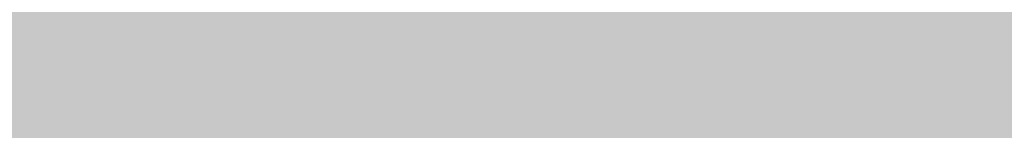
# Model space of a CAD drawing. Units: millimetres. Extents: x 0 to 2267, y 0 to 1823.
# Tile 243 of 256: x 1842.748 to 1843.095, y 1127.4234 to 1127.4624. Entities that reach past the tile are written whole.
import ezdxf

# ---------------------------------------------------------------- set-up
doc = ezdxf.new("R2010")
doc.units = ezdxf.units.MM
doc.header["$MEASUREMENT"] = 0
doc.layers.add('M-HATC', color=252, linetype='Continuous', lineweight=18)

msp = doc.modelspace()

# ---------------------------------------------------------------- hatches: boundary and pattern name
at = {"layer": 'M-HATC'}
h = msp.add_hatch(color=256, dxfattribs=at)
h.dxf.hatch_style = 1
h.paths.add_polyline_path([(2055.77105, 1603.06204), (1381.08677, 1603.06204), (1381.08677, 1598.06204), (2055.77105, 1598.06204)])
h.paths.add_polyline_path([(2055.77105, 1598.06204), (1381.08677, 1598.06204), (1381.08677, 1593.06204), (2055.77105, 1593.06204)])
h.paths.add_polyline_path([(2051.30737, 1536.76088), (1385.55044, 1536.76088), (1385.55044, 1526.76088), (1387.55044, 1526.76088), (1388.53662, 1525.05276), (1385.33187, 1521.23348), (1385.33187, 1521.22256), (2050.25417, 1522.74913), (2048.32119, 1525.05276), (2049.30737, 1526.76088), (2051.30737, 1526.76088)])
edge = h.paths.add_edge_path()
edge.add_arc((1847.53451, 1379.14917), 135, 222.6030607, 222.8908505, ccw=False)
edge.add_line((1748.16629, 1287.76561), (1683.09212, 1287.76561))
edge.add_arc((1583.7239, 1379.14917), 135, 317.1091495, 317.3969393, ccw=False)
edge.add_arc((1678.9686, 1290.67067), 5, 222.89085, 317.10915, ccw=False)
edge.add_arc((1774.21331, 1379.14917), 135, 222.6030607, 222.8908505, ccw=False)
edge.add_line((1674.84509, 1287.76561), (1609.77092, 1287.76561))
edge.add_arc((1510.4027, 1379.14917), 135, 317.1091495, 317.3969393, ccw=False)
edge.add_arc((1605.6474, 1290.67067), 5, 222.89085, 317.10915, ccw=False)
edge.add_arc((1700.89211, 1379.14917), 135, 222.6030607, 222.8908505, ccw=False)
edge.add_line((1601.52388, 1287.76561), (1536.44972, 1287.76561))
edge.add_arc((1437.08149, 1379.14917), 135, 317.1091495, 317.3969393, ccw=False)
edge.add_arc((1532.3262, 1290.67067), 5, 222.89085, 317.10915, ccw=False)
edge.add_arc((1627.57091, 1379.14917), 135, 222.6030607, 222.8908505, ccw=False)
edge.add_line((1528.20268, 1287.76561), (1505.92891, 1287.76561))
edge.add_spline(control_points=[(1505.92891, 1287.76561), (1504.26224, 1287.76561), (1504.26224, 1282.76561), (1505.92891, 1282.76561)], knot_values=[0, 0, 0, 0, 5, 5, 5, 5], degree=3, periodic=0)
edge.add_line((1505.92891, 1282.76561), (1930.92891, 1282.76561))
edge.add_spline(control_points=[(1930.92891, 1282.76561), (1932.59557, 1282.76561), (1932.59557, 1287.76561), (1930.92891, 1287.76561)], knot_values=[0, 0, 0, 0, 5, 5, 5, 5], degree=3, periodic=0)
edge.add_line((1930.92891, 1287.76561), (1903.05573, 1287.76561))
edge.add_arc((1803.6875, 1379.14917), 135, 317.1091495, 317.3969393, ccw=False)
edge.add_arc((1898.93221, 1290.67067), 5, 222.89085, 317.10915, ccw=False)
edge.add_arc((1994.17691, 1379.14917), 135, 222.6030607, 222.8908505, ccw=False)
edge.add_line((1894.80869, 1287.76561), (1829.73452, 1287.76561))
edge.add_arc((1730.3663, 1379.14917), 135, 317.1091495, 317.3969393, ccw=False)
edge.add_arc((1825.61101, 1290.67067), 5, 222.89085, 317.10915, ccw=False)
edge.add_arc((1920.85571, 1379.14917), 135, 222.6030607, 222.8908505, ccw=False)
edge.add_line((1821.48749, 1287.76561), (1756.41332, 1287.76561))
edge.add_arc((1657.0451, 1379.14917), 135, 317.1091495, 317.3969393, ccw=False)
edge.add_arc((1752.28981, 1290.67067), 5, 222.89085, 317.10915, ccw=False)
edge = h.paths.add_edge_path()
edge.add_spline(control_points=[(1843.42891, 1227.24746), (1845.09557, 1227.24746), (1845.09557, 1232.24746), (1843.42891, 1232.24746)], knot_values=[0, 0, 0, 0, 5, 5, 5, 5], degree=3, periodic=0)
edge.add_line((1843.42891, 1232.24746), (1593.42891, 1232.24746))
edge.add_spline(control_points=[(1593.42891, 1232.24746), (1591.76224, 1232.24746), (1591.76224, 1227.24746), (1593.42891, 1227.24746)], knot_values=[0, 0, 0, 0, 5, 5, 5, 5], degree=3, periodic=0)
edge.add_line((1593.42891, 1227.24746), (1843.42891, 1227.24746))
h.paths.add_polyline_path([(1905.92891, 1127.41706), (1530.92891, 1127.41706, 0.414214), (1520.92891, 1117.41706), (1530.92891, 1117.41706), (1915.92891, 1117.41706, 0.414214)])
edge = h.paths.add_edge_path()
edge.add_arc((1397.08577, 1498.40775), 12.72993, 90.782146, 190.878706, ccw=False)
edge.add_line((1396.912, 1511.13649), (1428.00968, 1511.34875))
edge.add_line((1428.00968, 1511.34875), (1433.00968, 1511.34875))
edge.add_line((1433.00968, 1511.34875), (1434.439, 1511.34875))
edge.add_arc((1419.474, 1498.08041), 20, 41.560995, 74.082109)
edge.add_line((1424.95919, 1517.31353), (1399.93509, 1517.25608))
edge.add_spline(control_points=[(1399.93074, 1517.25607), (1399.88398, 1517.21312), (1399.8328, 1517.16893), (1399.77741, 1517.1236)], knot_values=[11.567499, 11.567499, 11.567499, 11.567499, 11.814249, 11.814249, 11.814249, 11.814249], degree=3, periodic=0)
edge.add_spline(control_points=[(1399.63279, 1517.00986), (1399.58305, 1516.97214), (1399.53072, 1516.93375), (1399.47591, 1516.89474)], knot_values=[11.167718, 11.167718, 11.167718, 11.167718, 11.365188, 11.365188, 11.365188, 11.365188], degree=3, periodic=0)
edge.add_spline(control_points=[(1399.33981, 1516.80007), (1399.15144, 1516.67185), (1398.93836, 1516.5377), (1398.70404, 1516.39942)], knot_values=[10.376405, 10.376405, 10.376405, 10.376405, 11.00994, 11.00994, 11.00994, 11.00994], degree=3, periodic=0)
edge.add_spline(control_points=[(1398.65716, 1516.37187), (1398.57885, 1516.32602), (1398.49825, 1516.27974), (1398.41549, 1516.23309)], knot_values=[10.125175, 10.125175, 10.125175, 10.125175, 10.334406, 10.334406, 10.334406, 10.334406], degree=3, periodic=0)
edge.add_spline(control_points=[(1398.26422, 1516.14874), (1398.19595, 1516.11107), (1398.12634, 1516.07319), (1398.05546, 1516.03513)], knot_values=[9.832246, 9.832246, 9.832246, 9.832246, 9.999658, 9.999658, 9.999658, 9.999658], degree=3, periodic=0)
edge.add_spline(control_points=[(1397.9987, 1516.00476), (1397.73115, 1515.86211), (1397.44602, 1515.71707), (1397.14664, 1515.57138)], knot_values=[9.161808, 9.161808, 9.161808, 9.161808, 9.787769, 9.787769, 9.787769, 9.787769], degree=3, periodic=0)
edge.add_spline(control_points=[(1397.14664, 1515.57138), (1396.84182, 1515.42305), (1396.52223, 1515.27404), (1396.1914, 1515.12621)], knot_values=[8.524455, 8.524455, 8.524455, 8.524455, 9.161808, 9.161808, 9.161808, 9.161808], degree=3, periodic=0)
edge.add_spline(control_points=[(1396.07771, 1515.07565), (1395.98538, 1515.03478), (1395.89222, 1514.99402), (1395.7983, 1514.9534)], knot_values=[8.275193, 8.275193, 8.275193, 8.275193, 8.451726, 8.451726, 8.451726, 8.451726], degree=3, periodic=0)
edge.add_spline(control_points=[(1395.60184, 1514.86912), (1395.49975, 1514.82568), (1395.39685, 1514.78244), (1395.29322, 1514.73944)], knot_values=[7.962917, 7.962917, 7.962917, 7.962917, 8.152764, 8.152764, 8.152764, 8.152764], degree=3, periodic=0)
edge.add_spline(control_points=[(1395.21158, 1514.70568), (1394.82779, 1514.5475), (1394.43452, 1514.39287), (1394.03645, 1514.24422)], knot_values=[7.21254, 7.21254, 7.21254, 7.21254, 7.913148, 7.913148, 7.913148, 7.913148], degree=3, periodic=0)
edge.add_spline(control_points=[(1394.03645, 1514.24422), (1393.70758, 1514.12142), (1393.37544, 1514.0027), (1393.04267, 1513.88945)], knot_values=[6.633733, 6.633733, 6.633733, 6.633733, 7.21254, 7.21254, 7.21254, 7.21254], degree=3, periodic=0)
edge.add_spline(control_points=[(1392.82142, 1513.81499), (1392.71978, 1513.78118), (1392.61815, 1513.74791), (1392.51658, 1513.71521)], knot_values=[6.328796, 6.328796, 6.328796, 6.328796, 6.505493, 6.505493, 6.505493, 6.505493], degree=3, periodic=0)
edge.add_spline(control_points=[(1392.51658, 1513.71521), (1392.31873, 1513.65151), (1392.12116, 1513.59001), (1391.92441, 1513.53098)], knot_values=[5.984605, 5.984605, 5.984605, 5.984605, 6.328796, 6.328796, 6.328796, 6.328796], degree=3, periodic=0)
edge.add_spline(control_points=[(1391.79155, 1513.49146), (1391.31215, 1513.35011), (1390.83842, 1513.22392), (1390.37844, 1513.11711)], knot_values=[5.066697, 5.066697, 5.066697, 5.066697, 5.907055, 5.907055, 5.907055, 5.907055], degree=3, periodic=0)
edge.add_spline(control_points=[(1390.37844, 1513.11711), (1390.17973, 1513.07097), (1389.98359, 1513.02845), (1389.79067, 1512.98988)], knot_values=[4.70367, 4.70367, 4.70367, 4.70367, 5.066695, 5.066695, 5.066695, 5.066695], degree=3, periodic=0)
edge.add_spline(control_points=[(1389.42203, 1512.92036), (1389.24588, 1512.88922), (1389.0729, 1512.86172), (1388.90364, 1512.83814)], knot_values=[4.130571, 4.130571, 4.130571, 4.130571, 4.469816, 4.469816, 4.469816, 4.469816], degree=3, periodic=0)
edge.add_spline(control_points=[(1388.90364, 1512.83814), (1388.59103, 1512.7946), (1388.29108, 1512.76444), (1388.00714, 1512.74941)], knot_values=[3.504031, 3.504031, 3.504031, 3.504031, 4.130571, 4.130571, 4.130571, 4.130571], degree=3, periodic=0)
edge.add_spline(control_points=[(1387.9356, 1512.74593), (1387.85378, 1512.74231), (1387.77334, 1512.73997), (1387.69435, 1512.73898)], knot_values=[3.268866, 3.268866, 3.268866, 3.268866, 3.451164, 3.451164, 3.451164, 3.451164], degree=3, periodic=0)
edge.add_spline(control_points=[(1387.33512, 1512.74426), (1387.20757, 1512.74991), (1387.08472, 1512.7597), (1386.96699, 1512.77385)], knot_values=[2.670686, 2.670686, 2.670686, 2.670686, 2.984, 2.984, 2.984, 2.984], degree=3, periodic=0)
edge.add_spline(control_points=[(1386.83274, 1512.79225), (1386.82093, 1512.79407), (1386.80917, 1512.79594), (1386.79747, 1512.79787)], knot_values=[2.516981, 2.516981, 2.516981, 2.516981, 2.549528, 2.549528, 2.549528, 2.549528], degree=3, periodic=0)
edge.add_spline(control_points=[(1386.45257, 1512.87348), (1386.42573, 1512.88105), (1386.39931, 1512.88895), (1386.3733, 1512.89719)], knot_values=[2.095869, 2.095869, 2.095869, 2.095869, 2.17941, 2.17941, 2.17941, 2.17941], degree=3, periodic=0)
edge.add_spline(control_points=[(1386.06911, 1513.01889), (1386.06338, 1513.02174), (1386.05768, 1513.02463), (1386.05201, 1513.02753)], knot_values=[1.72453, 1.72453, 1.72453, 1.72453, 1.745933, 1.745933, 1.745933, 1.745933], degree=3, periodic=0)
edge.add_arc((1399.474, 1498.08041), 20, 131.824322, 180)
edge.add_arc((1630.33362, 1505.54843), 250.97076, 181.7051759, 236.427975)
edge.add_arc((1605.33992, 1483.30441), 218.7822, 238.660829, 243.3496099)
edge.add_arc((1647.09105, 1510.35917), 262.89859, 183.1298361, 237.8534422, ccw=False)
h.paths.add_polyline_path([(1406.53685, 1391.96444, 0.149382), (1491.55061, 1296.44177, -0.129517)], flags=17)
edge = h.paths.add_edge_path()
edge.add_arc((2037.38381, 1498.08041), 20, 0, 48.265868)
edge.add_spline(control_points=[(2050.69731, 1513.00525), (2050.65121, 1512.98471), (2050.60338, 1512.96554), (2050.55388, 1512.94771)], knot_values=[1.835652, 1.835652, 1.835652, 1.835652, 2.000781, 2.000781, 2.000781, 2.000781], degree=3, periodic=0)
edge.add_spline(control_points=[(2050.46156, 1512.91661), (2050.479, 1512.9221), (2050.49625, 1512.92774), (2050.51332, 1512.93353)], knot_values=[2.045477, 2.045477, 2.045477, 2.045477, 2.101389, 2.101389, 2.101389, 2.101389], degree=3, periodic=0)
edge.add_spline(control_points=[(2050.12896, 1512.83416), (2050.19843, 1512.84734), (2050.26573, 1512.86233), (2050.33075, 1512.87919)], knot_values=[2.237629, 2.237629, 2.237629, 2.237629, 2.435841, 2.435841, 2.435841, 2.435841], degree=3, periodic=0)
edge.add_spline(control_points=[(2050.09463, 1512.82783), (2050.10613, 1512.82989), (2050.11757, 1512.832), (2050.12896, 1512.83416)], knot_values=[2.435841, 2.435841, 2.435841, 2.435841, 2.468321, 2.468321, 2.468321, 2.468321], degree=3, periodic=0)
edge.add_spline(control_points=[(2049.78433, 1512.78511), (2049.85521, 1512.79219), (2049.92435, 1512.80077), (2049.99166, 1512.81088)], knot_values=[2.563852, 2.563852, 2.563852, 2.563852, 2.748541, 2.748541, 2.748541, 2.748541], degree=3, periodic=0)
edge.add_spline(control_points=[(2049.4052, 1512.76169), (2049.5364, 1512.76526), (2049.66292, 1512.77299), (2049.78433, 1512.78511)], knot_values=[2.748541, 2.748541, 2.748541, 2.748541, 3.064882, 3.064882, 3.064882, 3.064882], degree=3, periodic=0)
edge.add_spline(control_points=[(2049.16976, 1512.75968), (2049.23364, 1512.7591), (2049.29654, 1512.7594), (2049.35844, 1512.7606)], knot_values=[3.102309, 3.102309, 3.102309, 3.102309, 3.2503, 3.2503, 3.2503, 3.2503], degree=3, periodic=0)
edge.add_spline(control_points=[(2048.85727, 1512.76911), (2048.96378, 1512.76378), (2049.068, 1512.76061), (2049.16976, 1512.75968)], knot_values=[3.2503, 3.2503, 3.2503, 3.2503, 3.486069, 3.486069, 3.486069, 3.486069], degree=3, periodic=0)
edge.add_spline(control_points=[(2048.69241, 1512.77892), (2048.3729, 1512.80093), (2048.0345, 1512.84106), (2047.68175, 1512.89697)], knot_values=[3.606429, 3.606429, 3.606429, 3.606429, 4.2989, 4.2989, 4.2989, 4.2989], degree=3, periodic=0)
edge.add_spline(control_points=[(2047.68175, 1512.89697), (2047.5458, 1512.91852), (2047.40772, 1512.94241), (2047.26776, 1512.96851)], knot_values=[4.2989, 4.2989, 4.2989, 4.2989, 4.565769, 4.565769, 4.565769, 4.565769], degree=3, periodic=0)
edge.add_spline(control_points=[(2047.26776, 1512.96851), (2047.14494, 1512.99141), (2047.02067, 1513.01601), (2046.89514, 1513.04223)], knot_values=[4.565769, 4.565769, 4.565769, 4.565769, 4.799971, 4.799971, 4.799971, 4.799971], degree=3, periodic=0)
edge.add_spline(control_points=[(2046.89514, 1513.04223), (2046.52865, 1513.11875), (2046.15135, 1513.20899), (2045.7676, 1513.31068)], knot_values=[4.799971, 4.799971, 4.799971, 4.799971, 5.483718, 5.483718, 5.483718, 5.483718], degree=3, periodic=0)
edge.add_spline(control_points=[(2045.7676, 1513.31068), (2045.3724, 1513.41539), (2044.97036, 1513.53225), (2044.56625, 1513.65876)], knot_values=[5.483718, 5.483718, 5.483718, 5.483718, 6.187866, 6.187866, 6.187866, 6.187866], degree=3, periodic=0)
edge.add_spline(control_points=[(2044.56625, 1513.65876), (2044.41491, 1513.70614), (2044.26329, 1513.75487), (2044.11163, 1513.80482)], knot_values=[6.187866, 6.187866, 6.187866, 6.187866, 6.451551, 6.451551, 6.451551, 6.451551], degree=3, periodic=0)
edge.add_spline(control_points=[(2044.11163, 1513.80482), (2043.99666, 1513.84269), (2043.88167, 1513.88126), (2043.76676, 1513.92048)], knot_values=[6.451551, 6.451551, 6.451551, 6.451551, 6.651434, 6.651434, 6.651434, 6.651434], degree=3, periodic=0)
edge.add_spline(control_points=[(2043.76676, 1513.92048), (2043.37157, 1514.05536), (2042.97738, 1514.19789), (2042.58863, 1514.34575)], knot_values=[6.651434, 6.651434, 6.651434, 6.651434, 7.338879, 7.338879, 7.338879, 7.338879], degree=3, periodic=0)
edge.add_spline(control_points=[(2042.58863, 1514.34575), (2042.16431, 1514.50715), (2041.74647, 1514.67491), (2041.34086, 1514.84603)], knot_values=[7.338879, 7.338879, 7.338879, 7.338879, 8.089209, 8.089209, 8.089209, 8.089209], degree=3, periodic=0)
edge.add_spline(control_points=[(2041.34086, 1514.84603), (2041.1028, 1514.94647), (2040.86896, 1515.04806), (2040.64049, 1515.1502)], knot_values=[8.089209, 8.089209, 8.089209, 8.089209, 8.529587, 8.529587, 8.529587, 8.529587], degree=3, periodic=0)
edge.add_spline(control_points=[(2040.50999, 1515.20887), (2040.08238, 1515.40218), (2039.67475, 1515.59705), (2039.29495, 1515.78939)], knot_values=[8.613818, 8.613818, 8.613818, 8.613818, 9.44571, 9.44571, 9.44571, 9.44571], degree=3, periodic=0)
edge.add_spline(control_points=[(2039.29495, 1515.78939), (2039.0618, 1515.90746), (2038.83914, 1516.02458), (2038.62878, 1516.1398)], knot_values=[9.44571, 9.44571, 9.44571, 9.44571, 9.956404, 9.956404, 9.956404, 9.956404], degree=3, periodic=0)
edge.add_spline(control_points=[(2038.62878, 1516.1398), (2038.51874, 1516.20007), (2038.41207, 1516.25982), (2038.30903, 1516.31891)], knot_values=[9.956404, 9.956404, 9.956404, 9.956404, 10.223542, 10.223542, 10.223542, 10.223542], degree=3, periodic=0)
edge.add_spline(control_points=[(2038.30903, 1516.31891), (2038.21377, 1516.37354), (2038.12161, 1516.42762), (2038.03275, 1516.48102)], knot_values=[10.223542, 10.223542, 10.223542, 10.223542, 10.47051, 10.47051, 10.47051, 10.47051], degree=3, periodic=0)
edge.add_spline(control_points=[(2038.03275, 1516.48102), (2037.78552, 1516.62961), (2037.56388, 1516.77304), (2037.37225, 1516.909)], knot_values=[10.47051, 10.47051, 10.47051, 10.47051, 11.15767, 11.15767, 11.15767, 11.15767], degree=3, periodic=0)
edge.add_spline(control_points=[(2037.37225, 1516.909), (2037.27893, 1516.9752), (2037.19274, 1517.03963), (2037.11417, 1517.10203)], knot_values=[11.15767, 11.15767, 11.15767, 11.15767, 11.49227, 11.49227, 11.49227, 11.49227], degree=3, periodic=0)
edge.add_spline(control_points=[(2036.85638, 1517.32585), (2036.91481, 1517.26923), (2036.98143, 1517.21027), (2037.05573, 1517.14922)], knot_values=[11.577341, 11.577341, 11.577341, 11.577341, 11.91035, 11.91035, 11.91035, 11.91035], degree=3, periodic=0)
edge.add_spline(control_points=[(2036.80739, 1517.37475), (2036.82301, 1517.35865), (2036.83935, 1517.34235), (2036.85638, 1517.32585)], knot_values=[11.91035, 11.91035, 11.91035, 11.91035, 12.007402, 12.007402, 12.007402, 12.007402], degree=3, periodic=0)
edge.add_spline(control_points=[(2036.70167, 1517.494), (2036.71042, 1517.48299), (2036.71958, 1517.47185), (2036.72913, 1517.4606)], knot_values=[12.184155, 12.184155, 12.184155, 12.184155, 12.255409, 12.255409, 12.255409, 12.255409], degree=3, periodic=0)
edge.add_spline(control_points=[(2036.6159, 1517.6205), (2036.61998, 1517.61304), (2036.6243, 1517.6055), (2036.62885, 1517.59789)], knot_values=[12.487913, 12.487913, 12.487913, 12.487913, 12.541035, 12.541035, 12.541035, 12.541035], degree=3, periodic=0)
edge.add_spline(control_points=[(2036.56349, 1517.78599), (2036.56372, 1517.77936), (2036.56423, 1517.77264), (2036.56502, 1517.76582)], knot_values=[12.911761, 12.911761, 12.911761, 12.911761, 12.968286, 12.968286, 12.968286, 12.968286], degree=3, periodic=0)
edge.add_spline(control_points=[(2036.61663, 1517.93042), (2036.61248, 1517.92586), (2036.60857, 1517.92121), (2036.60491, 1517.91648)], knot_values=[13.382527, 13.382527, 13.382527, 13.382527, 13.433791, 13.433791, 13.433791, 13.433791], degree=3, periodic=0)
edge.add_spline(control_points=[(2036.74902, 1518.01695), (2036.73613, 1518.0116), (2036.72393, 1518.00601), (2036.71242, 1518.00018)], knot_values=[13.726299, 13.726299, 13.726299, 13.726299, 13.809928, 13.809928, 13.809928, 13.809928], degree=3, periodic=0)
edge.add_spline(control_points=[(2036.86043, 1518.05285), (2036.83863, 1518.04743), (2036.81809, 1518.04156), (2036.79879, 1518.03526)], knot_values=[13.910887, 13.910887, 13.910887, 13.910887, 14.02153, 14.02153, 14.02153, 14.02153], degree=3, periodic=0)
edge.add_line((2036.96387, 1518.08041), (2032.38381, 1518.08041))
edge.add_line((2032.38381, 1518.08041), (2027.38381, 1518.08041))
edge.add_line((2027.38381, 1518.08041), (2022.38381, 1518.08041))
edge.add_line((2022.38381, 1518.08041), (2017.38381, 1518.08041))
edge.add_arc((2017.38381, 1498.08041), 20, 90, 138.439005)
edge.add_line((2002.41881, 1511.34875), (2003.84813, 1511.34875))
edge.add_line((2003.84813, 1511.34875), (2008.84813, 1511.34875))
edge.add_line((2008.84813, 1511.34875), (2039.77204, 1511.13768))
edge.add_arc((2039.77204, 1498.40775), 12.72993, -10.878706, 90, ccw=False)
edge.add_arc((1789.76676, 1510.35917), 262.89859, 302.1465578, 356.8701639, ccw=False)
edge.add_arc((1831.51789, 1483.30441), 218.7822, 296.6503901, 301.339171)
edge.add_arc((1806.52419, 1505.54843), 250.97076, 303.572025, 358.2948241)
h.paths.add_polyline_path([(2030.32096, 1391.96444, -0.129517), (1945.3072, 1296.44177, 0.149382)], flags=17)
edge = h.paths.add_edge_path()
edge.add_spline(control_points=[(2037.2464, 1518.08209), (2037.28977, 1518.08098), (2037.33555, 1518.08041), (2037.3838, 1518.08041)], knot_values=[0.000012, 0.000012, 0.000012, 0.000012, 0.144754, 0.144754, 0.144754, 0.144754], degree=3, periodic=0)
edge.add_line((2037.33571, 1518.08041), (2037.00963, 1518.08041))
edge.add_spline(control_points=[(2037.00963, 1518.08041), (2036.98217, 1518.07678), (2036.95605, 1518.07266), (2036.93124, 1518.06808)], knot_values=[14.13465, 14.13465, 14.13465, 14.13465, 14.247197, 14.247197, 14.247197, 14.247197], degree=3, periodic=0)
edge.add_spline(control_points=[(2036.93124, 1518.06808), (2036.92764, 1518.06741), (2036.92407, 1518.06674), (2036.92053, 1518.06605)], knot_values=[14.118315, 14.118315, 14.118315, 14.118315, 14.13465, 14.13465, 14.13465, 14.13465], degree=3, periodic=0)
edge.add_spline(control_points=[(2036.92053, 1518.06605), (2036.9118, 1518.06436), (2036.90323, 1518.06262), (2036.89484, 1518.06081)], knot_values=[14.078086, 14.078086, 14.078086, 14.078086, 14.118315, 14.118315, 14.118315, 14.118315], degree=3, periodic=0)
edge.add_spline(control_points=[(2036.89484, 1518.06081), (2036.88304, 1518.05827), (2036.87157, 1518.05562), (2036.86043, 1518.05285)], knot_values=[14.02153, 14.02153, 14.02153, 14.02153, 14.078086, 14.078086, 14.078086, 14.078086], degree=3, periodic=0)
edge.add_spline(control_points=[(2036.86043, 1518.05285), (2036.83863, 1518.04743), (2036.81809, 1518.04156), (2036.79879, 1518.03526)], knot_values=[13.910887, 13.910887, 13.910887, 13.910887, 14.02153, 14.02153, 14.02153, 14.02153], degree=3, periodic=0)
edge.add_spline(control_points=[(2036.79879, 1518.03526), (2036.79809, 1518.03504), (2036.7974, 1518.03481), (2036.79671, 1518.03458)], knot_values=[13.906906, 13.906906, 13.906906, 13.906906, 13.910887, 13.910887, 13.910887, 13.910887], degree=3, periodic=0)
edge.add_spline(control_points=[(2036.79671, 1518.03458), (2036.78819, 1518.03178), (2036.77991, 1518.02888), (2036.77187, 1518.02591)], knot_values=[13.857826, 13.857826, 13.857826, 13.857826, 13.906906, 13.906906, 13.906906, 13.906906], degree=3, periodic=0)
edge.add_spline(control_points=[(2036.77187, 1518.02591), (2036.76402, 1518.023), (2036.75641, 1518.02002), (2036.74902, 1518.01695)], knot_values=[13.809928, 13.809928, 13.809928, 13.809928, 13.857826, 13.857826, 13.857826, 13.857826], degree=3, periodic=0)
edge.add_spline(control_points=[(2036.74902, 1518.01695), (2036.73613, 1518.0116), (2036.72393, 1518.00601), (2036.71242, 1518.00018)], knot_values=[13.726299, 13.726299, 13.726299, 13.726299, 13.809928, 13.809928, 13.809928, 13.809928], degree=3, periodic=0)
edge.add_spline(control_points=[(2036.71242, 1518.00018), (2036.71211, 1518.00002), (2036.71179, 1517.99986), (2036.71147, 1517.99969)], knot_values=[13.723993, 13.723993, 13.723993, 13.723993, 13.726299, 13.726299, 13.726299, 13.726299], degree=3, periodic=0)
edge.add_spline(control_points=[(2036.71147, 1517.99969), (2036.70634, 1517.99708), (2036.70134, 1517.99441), (2036.69648, 1517.9917)], knot_values=[13.686536, 13.686536, 13.686536, 13.686536, 13.723993, 13.723993, 13.723993, 13.723993], degree=3, periodic=0)
edge.add_spline(control_points=[(2036.69648, 1517.9917), (2036.6919, 1517.98914), (2036.68744, 1517.98654), (2036.6831, 1517.9839)], knot_values=[13.651251, 13.651251, 13.651251, 13.651251, 13.686536, 13.686536, 13.686536, 13.686536], degree=3, periodic=0)
edge.add_spline(control_points=[(2036.6831, 1517.9839), (2036.67641, 1517.97983), (2036.67001, 1517.97566), (2036.6639, 1517.97139)], knot_values=[13.596804, 13.596804, 13.596804, 13.596804, 13.651251, 13.651251, 13.651251, 13.651251], degree=3, periodic=0)
edge.add_spline(control_points=[(2036.6639, 1517.97139), (2036.66358, 1517.97117), (2036.66326, 1517.97094), (2036.66294, 1517.97072)], knot_values=[13.593956, 13.593956, 13.593956, 13.593956, 13.596804, 13.596804, 13.596804, 13.596804], degree=3, periodic=0)
edge.add_spline(control_points=[(2036.66294, 1517.97072), (2036.6603, 1517.96886), (2036.65771, 1517.96698), (2036.65518, 1517.96509)], knot_values=[13.570322, 13.570322, 13.570322, 13.570322, 13.593956, 13.593956, 13.593956, 13.593956], degree=3, periodic=0)
edge.add_spline(control_points=[(2036.65518, 1517.96509), (2036.65251, 1517.9631), (2036.64991, 1517.96108), (2036.64737, 1517.95905)], knot_values=[13.545477, 13.545477, 13.545477, 13.545477, 13.570322, 13.570322, 13.570322, 13.570322], degree=3, periodic=0)
edge.add_spline(control_points=[(2036.64737, 1517.95905), (2036.64721, 1517.95892), (2036.64705, 1517.9588), (2036.64689, 1517.95867)], knot_values=[13.543931, 13.543931, 13.543931, 13.543931, 13.545477, 13.545477, 13.545477, 13.545477], degree=3, periodic=0)
edge.add_spline(control_points=[(2036.64689, 1517.95867), (2036.64121, 1517.95411), (2036.63582, 1517.94945), (2036.63073, 1517.94468)], knot_values=[13.488237, 13.488237, 13.488237, 13.488237, 13.543931, 13.543931, 13.543931, 13.543931], degree=3, periodic=0)
edge.add_spline(control_points=[(2036.63073, 1517.94468), (2036.62817, 1517.94229), (2036.62569, 1517.93988), (2036.62329, 1517.93744)], knot_values=[13.460307, 13.460307, 13.460307, 13.460307, 13.488237, 13.488237, 13.488237, 13.488237], degree=3, periodic=0)
edge.add_spline(control_points=[(2036.62329, 1517.93744), (2036.62151, 1517.93564), (2036.61978, 1517.93383), (2036.61809, 1517.932)], knot_values=[13.439712, 13.439712, 13.439712, 13.439712, 13.460307, 13.460307, 13.460307, 13.460307], degree=3, periodic=0)
edge.add_spline(control_points=[(2036.61809, 1517.932), (2036.6176, 1517.93147), (2036.61711, 1517.93095), (2036.61663, 1517.93042)], knot_values=[13.433791, 13.433791, 13.433791, 13.433791, 13.439712, 13.439712, 13.439712, 13.439712], degree=3, periodic=0)
edge.add_spline(control_points=[(2036.61663, 1517.93042), (2036.61248, 1517.92586), (2036.60857, 1517.92121), (2036.60491, 1517.91648)], knot_values=[13.382527, 13.382527, 13.382527, 13.382527, 13.433791, 13.433791, 13.433791, 13.433791], degree=3, periodic=0)
edge.add_spline(control_points=[(2036.60491, 1517.91648), (2036.60258, 1517.91347), (2036.60036, 1517.91044), (2036.59824, 1517.90737)], knot_values=[13.350017, 13.350017, 13.350017, 13.350017, 13.382527, 13.382527, 13.382527, 13.382527], degree=3, periodic=0)
edge.add_spline(control_points=[(2036.59824, 1517.90737), (2036.59718, 1517.90585), (2036.59616, 1517.90433), (2036.59515, 1517.90279)], knot_values=[13.333922, 13.333922, 13.333922, 13.333922, 13.350017, 13.350017, 13.350017, 13.350017], degree=3, periodic=0)
edge.add_spline(control_points=[(2036.59515, 1517.90279), (2036.59452, 1517.90183), (2036.5939, 1517.90086), (2036.59329, 1517.89989)], knot_values=[13.323828, 13.323828, 13.323828, 13.323828, 13.333922, 13.333922, 13.333922, 13.333922], degree=3, periodic=0)
edge.add_spline(control_points=[(2036.59329, 1517.89989), (2036.59049, 1517.89545), (2036.5879, 1517.89094), (2036.5855, 1517.88637)], knot_values=[13.277545, 13.277545, 13.277545, 13.277545, 13.323828, 13.323828, 13.323828, 13.323828], degree=3, periodic=0)
edge.add_spline(control_points=[(2036.5855, 1517.88637), (2036.58355, 1517.88267), (2036.58174, 1517.87892), (2036.58006, 1517.87513)], knot_values=[13.240119, 13.240119, 13.240119, 13.240119, 13.277545, 13.277545, 13.277545, 13.277545], degree=3, periodic=0)
edge.add_spline(control_points=[(2036.58006, 1517.87513), (2036.57952, 1517.87393), (2036.579, 1517.87272), (2036.57849, 1517.87151)], knot_values=[13.228211, 13.228211, 13.228211, 13.228211, 13.240119, 13.240119, 13.240119, 13.240119], degree=3, periodic=0)
edge.add_spline(control_points=[(2036.57849, 1517.87151), (2036.57796, 1517.87023), (2036.57744, 1517.86896), (2036.57693, 1517.86767)], knot_values=[13.215717, 13.215717, 13.215717, 13.215717, 13.228211, 13.228211, 13.228211, 13.228211], degree=3, periodic=0)
edge.add_spline(control_points=[(2036.57693, 1517.86767), (2036.57548, 1517.86399), (2036.57414, 1517.86027), (2036.57293, 1517.85651)], knot_values=[13.179847, 13.179847, 13.179847, 13.179847, 13.215717, 13.215717, 13.215717, 13.215717], degree=3, periodic=0)
edge.add_spline(control_points=[(2036.57293, 1517.85651), (2036.5713, 1517.8515), (2036.56989, 1517.84641), (2036.56868, 1517.84126)], knot_values=[13.132017, 13.132017, 13.132017, 13.132017, 13.179847, 13.179847, 13.179847, 13.179847], degree=3, periodic=0)
edge.add_spline(control_points=[(2036.56868, 1517.84126), (2036.56844, 1517.84023), (2036.56821, 1517.8392), (2036.56798, 1517.83817)], knot_values=[13.122482, 13.122482, 13.122482, 13.122482, 13.132017, 13.132017, 13.132017, 13.132017], degree=3, periodic=0)
edge.add_spline(control_points=[(2036.56798, 1517.83817), (2036.56758, 1517.83634), (2036.56721, 1517.8345), (2036.56687, 1517.83266)], knot_values=[13.105592, 13.105592, 13.105592, 13.105592, 13.122482, 13.122482, 13.122482, 13.122482], degree=3, periodic=0)
edge.add_spline(control_points=[(2036.56687, 1517.83266), (2036.56622, 1517.82921), (2036.56567, 1517.82574), (2036.5652, 1517.82223)], knot_values=[13.074063, 13.074063, 13.074063, 13.074063, 13.105592, 13.105592, 13.105592, 13.105592], degree=3, periodic=0)
edge.add_spline(control_points=[(2036.5652, 1517.82223), (2036.5652, 1517.82223), (2036.5652, 1517.82223), (2036.5652, 1517.82223)], knot_values=[13.074043, 13.074043, 13.074043, 13.074043, 13.074063, 13.074063, 13.074063, 13.074063], degree=3, periodic=0)
edge.add_spline(control_points=[(2036.5652, 1517.82223), (2036.56443, 1517.81643), (2036.5639, 1517.81055), (2036.56361, 1517.8046)], knot_values=[13.021884, 13.021884, 13.021884, 13.021884, 13.074043, 13.074043, 13.074043, 13.074043], degree=3, periodic=0)
edge.add_spline(control_points=[(2036.56361, 1517.8046), (2036.56358, 1517.80401), (2036.56356, 1517.80342), (2036.56353, 1517.80283)], knot_values=[13.01674, 13.01674, 13.01674, 13.01674, 13.021884, 13.021884, 13.021884, 13.021884], degree=3, periodic=0)
edge.add_spline(control_points=[(2036.56353, 1517.80283), (2036.56344, 1517.80051), (2036.56338, 1517.79817), (2036.56336, 1517.79582)], knot_values=[12.996438, 12.996438, 12.996438, 12.996438, 13.01674, 13.01674, 13.01674, 13.01674], degree=3, periodic=0)
edge.add_spline(control_points=[(2036.56336, 1517.79582), (2036.56334, 1517.79257), (2036.56338, 1517.78929), (2036.56349, 1517.78599)], knot_values=[12.968286, 12.968286, 12.968286, 12.968286, 12.996438, 12.996438, 12.996438, 12.996438], degree=3, periodic=0)
edge.add_spline(control_points=[(2036.56349, 1517.78599), (2036.56372, 1517.77936), (2036.56423, 1517.77264), (2036.56502, 1517.76582)], knot_values=[12.911761, 12.911761, 12.911761, 12.911761, 12.968286, 12.968286, 12.968286, 12.968286], degree=3, periodic=0)
edge.add_spline(control_points=[(2036.56502, 1517.76582), (2036.56503, 1517.76573), (2036.56504, 1517.76564), (2036.56505, 1517.76555)], knot_values=[12.911017, 12.911017, 12.911017, 12.911017, 12.911761, 12.911761, 12.911761, 12.911761], degree=3, periodic=0)
edge.add_spline(control_points=[(2036.56505, 1517.76555), (2036.56541, 1517.76245), (2036.56583, 1517.75933), (2036.56631, 1517.75619)], knot_values=[12.88528, 12.88528, 12.88528, 12.88528, 12.911017, 12.911017, 12.911017, 12.911017], degree=3, periodic=0)
edge.add_spline(control_points=[(2036.56631, 1517.75619), (2036.56673, 1517.75341), (2036.5672, 1517.75062), (2036.56771, 1517.74782)], knot_values=[12.862519, 12.862519, 12.862519, 12.862519, 12.88528, 12.88528, 12.88528, 12.88528], degree=3, periodic=0)
edge.add_spline(control_points=[(2036.56771, 1517.74782), (2036.56779, 1517.74737), (2036.56788, 1517.74692), (2036.56796, 1517.74647)], knot_values=[12.858885, 12.858885, 12.858885, 12.858885, 12.862519, 12.862519, 12.862519, 12.862519], degree=3, periodic=0)
edge.add_spline(control_points=[(2036.56796, 1517.74647), (2036.5692, 1517.73986), (2036.57069, 1517.73316), (2036.57243, 1517.72638)], knot_values=[12.8053, 12.8053, 12.8053, 12.8053, 12.858885, 12.858885, 12.858885, 12.858885], degree=3, periodic=0)
edge.add_spline(control_points=[(2036.57243, 1517.72638), (2036.5734, 1517.72257), (2036.57446, 1517.71874), (2036.57559, 1517.71488)], knot_values=[12.775176, 12.775176, 12.775176, 12.775176, 12.8053, 12.8053, 12.8053, 12.8053], degree=3, periodic=0)
edge.add_spline(control_points=[(2036.57559, 1517.71488), (2036.57628, 1517.71252), (2036.577, 1517.71015), (2036.57775, 1517.70778)], knot_values=[12.756759, 12.756759, 12.756759, 12.756759, 12.775176, 12.775176, 12.775176, 12.775176], degree=3, periodic=0)
edge.add_spline(control_points=[(2036.57775, 1517.70778), (2036.57808, 1517.70674), (2036.57841, 1517.7057), (2036.57875, 1517.70466)], knot_values=[12.748742, 12.748742, 12.748742, 12.748742, 12.756759, 12.756759, 12.756759, 12.756759], degree=3, periodic=0)
edge.add_spline(control_points=[(2036.57875, 1517.70466), (2036.58082, 1517.6983), (2036.58309, 1517.69187), (2036.58557, 1517.68537)], knot_values=[12.69959, 12.69959, 12.69959, 12.69959, 12.748742, 12.748742, 12.748742, 12.748742], degree=3, periodic=0)
edge.add_spline(control_points=[(2036.58557, 1517.68537), (2036.58762, 1517.68001), (2036.5898, 1517.6746), (2036.59213, 1517.66916)], knot_values=[12.659038, 12.659038, 12.659038, 12.659038, 12.69959, 12.69959, 12.69959, 12.69959], degree=3, periodic=0)
edge.add_spline(control_points=[(2036.59213, 1517.66916), (2036.59397, 1517.66482), (2036.59591, 1517.66047), (2036.59793, 1517.65608)], knot_values=[12.626806, 12.626806, 12.626806, 12.626806, 12.659038, 12.659038, 12.659038, 12.659038], degree=3, periodic=0)
edge.add_spline(control_points=[(2036.59793, 1517.65608), (2036.59839, 1517.65507), (2036.59886, 1517.65406), (2036.59934, 1517.65305)], knot_values=[12.619394, 12.619394, 12.619394, 12.619394, 12.626806, 12.626806, 12.626806, 12.626806], degree=3, periodic=0)
edge.add_spline(control_points=[(2036.59934, 1517.65305), (2036.60435, 1517.64236), (2036.60987, 1517.63151), (2036.61589, 1517.6205)], knot_values=[12.541039, 12.541039, 12.541039, 12.541039, 12.619394, 12.619394, 12.619394, 12.619394], degree=3, periodic=0)
edge.add_spline(control_points=[(2036.61589, 1517.6205), (2036.61589, 1517.6205), (2036.6159, 1517.6205), (2036.6159, 1517.6205)], knot_values=[12.541035, 12.541035, 12.541035, 12.541035, 12.541039, 12.541039, 12.541039, 12.541039], degree=3, periodic=0)
edge.add_spline(control_points=[(2036.6159, 1517.6205), (2036.61998, 1517.61304), (2036.6243, 1517.6055), (2036.62885, 1517.59789)], knot_values=[12.487913, 12.487913, 12.487913, 12.487913, 12.541035, 12.541035, 12.541035, 12.541035], degree=3, periodic=0)
edge.add_spline(control_points=[(2036.62885, 1517.59789), (2036.63261, 1517.5916), (2036.63653, 1517.58526), (2036.64061, 1517.57888)], knot_values=[12.443982, 12.443982, 12.443982, 12.443982, 12.487913, 12.487913, 12.487913, 12.487913], degree=3, periodic=0)
edge.add_spline(control_points=[(2036.64061, 1517.57888), (2036.64144, 1517.57757), (2036.64228, 1517.57626), (2036.64313, 1517.57495)], knot_values=[12.434996, 12.434996, 12.434996, 12.434996, 12.443982, 12.443982, 12.443982, 12.443982], degree=3, periodic=0)
edge.add_spline(control_points=[(2036.64313, 1517.57495), (2036.65306, 1517.55958), (2036.66389, 1517.54394), (2036.6756, 1517.52803)], knot_values=[12.329647, 12.329647, 12.329647, 12.329647, 12.434996, 12.434996, 12.434996, 12.434996], degree=3, periodic=0)
edge.add_spline(control_points=[(2036.6756, 1517.52803), (2036.68385, 1517.51682), (2036.69254, 1517.50548), (2036.70167, 1517.494)], knot_values=[12.255409, 12.255409, 12.255409, 12.255409, 12.329647, 12.329647, 12.329647, 12.329647], degree=3, periodic=0)
edge.add_spline(control_points=[(2036.70167, 1517.494), (2036.71042, 1517.48299), (2036.71958, 1517.47185), (2036.72913, 1517.4606)], knot_values=[12.184155, 12.184155, 12.184155, 12.184155, 12.255409, 12.255409, 12.255409, 12.255409], degree=3, periodic=0)
edge.add_spline(control_points=[(2036.72913, 1517.4606), (2036.74363, 1517.44352), (2036.75904, 1517.42617), (2036.77534, 1517.40855)], knot_values=[12.075961, 12.075961, 12.075961, 12.075961, 12.184155, 12.184155, 12.184155, 12.184155], degree=3, periodic=0)
edge.add_spline(control_points=[(2036.77534, 1517.40855), (2036.77631, 1517.4075), (2036.77729, 1517.40645), (2036.77827, 1517.40539)], knot_values=[12.069502, 12.069502, 12.069502, 12.069502, 12.075961, 12.075961, 12.075961, 12.075961], degree=3, periodic=0)
edge.add_spline(control_points=[(2036.77827, 1517.40539), (2036.78768, 1517.39526), (2036.79739, 1517.38505), (2036.80739, 1517.37475)], knot_values=[12.007402, 12.007402, 12.007402, 12.007402, 12.069502, 12.069502, 12.069502, 12.069502], degree=3, periodic=0)
edge.add_spline(control_points=[(2036.80739, 1517.37475), (2036.82301, 1517.35865), (2036.83935, 1517.34235), (2036.85638, 1517.32585)], knot_values=[11.91035, 11.91035, 11.91035, 11.91035, 12.007402, 12.007402, 12.007402, 12.007402], degree=3, periodic=0)
edge.add_spline(control_points=[(2036.85638, 1517.32585), (2036.91481, 1517.26923), (2036.98143, 1517.21027), (2037.05573, 1517.14922)], knot_values=[11.577341, 11.577341, 11.577341, 11.577341, 11.91035, 11.91035, 11.91035, 11.91035], degree=3, periodic=0)
edge.add_spline(control_points=[(2037.05573, 1517.14922), (2037.07471, 1517.13362), (2037.0942, 1517.11789), (2037.11417, 1517.10203)], knot_values=[11.49227, 11.49227, 11.49227, 11.49227, 11.577341, 11.577341, 11.577341, 11.577341], degree=3, periodic=0)
edge.add_spline(control_points=[(2037.11417, 1517.10203), (2037.19274, 1517.03963), (2037.27893, 1516.9752), (2037.37225, 1516.909)], knot_values=[11.15767, 11.15767, 11.15767, 11.15767, 11.49227, 11.49227, 11.49227, 11.49227], degree=3, periodic=0)
edge.add_spline(control_points=[(2037.37225, 1516.909), (2037.56388, 1516.77304), (2037.78552, 1516.62961), (2038.03275, 1516.48102)], knot_values=[10.47051, 10.47051, 10.47051, 10.47051, 11.15767, 11.15767, 11.15767, 11.15767], degree=3, periodic=0)
edge.add_spline(control_points=[(2038.03275, 1516.48102), (2038.12161, 1516.42762), (2038.21377, 1516.37354), (2038.30903, 1516.31891)], knot_values=[10.223542, 10.223542, 10.223542, 10.223542, 10.47051, 10.47051, 10.47051, 10.47051], degree=3, periodic=0)
edge.add_spline(control_points=[(2038.30903, 1516.31891), (2038.41207, 1516.25982), (2038.51874, 1516.20007), (2038.62878, 1516.1398)], knot_values=[9.956404, 9.956404, 9.956404, 9.956404, 10.223542, 10.223542, 10.223542, 10.223542], degree=3, periodic=0)
edge.add_spline(control_points=[(2038.62878, 1516.1398), (2038.83914, 1516.02458), (2039.0618, 1515.90746), (2039.29495, 1515.78939)], knot_values=[9.44571, 9.44571, 9.44571, 9.44571, 9.956404, 9.956404, 9.956404, 9.956404], degree=3, periodic=0)
edge.add_spline(control_points=[(2039.29495, 1515.78939), (2039.67475, 1515.59705), (2040.08238, 1515.40218), (2040.50999, 1515.20887)], knot_values=[8.613818, 8.613818, 8.613818, 8.613818, 9.44571, 9.44571, 9.44571, 9.44571], degree=3, periodic=0)
edge.add_spline(control_points=[(2040.50999, 1515.20887), (2040.55329, 1515.1893), (2040.59679, 1515.16974), (2040.64049, 1515.1502)], knot_values=[8.529587, 8.529587, 8.529587, 8.529587, 8.613818, 8.613818, 8.613818, 8.613818], degree=3, periodic=0)
edge.add_spline(control_points=[(2040.64049, 1515.1502), (2040.86896, 1515.04806), (2041.1028, 1514.94647), (2041.34086, 1514.84603)], knot_values=[8.089209, 8.089209, 8.089209, 8.089209, 8.529587, 8.529587, 8.529587, 8.529587], degree=3, periodic=0)
edge.add_spline(control_points=[(2041.34086, 1514.84603), (2041.74647, 1514.67491), (2042.16431, 1514.50715), (2042.58863, 1514.34575)], knot_values=[7.338879, 7.338879, 7.338879, 7.338879, 8.089209, 8.089209, 8.089209, 8.089209], degree=3, periodic=0)
edge.add_spline(control_points=[(2042.58863, 1514.34575), (2042.97738, 1514.19789), (2043.37157, 1514.05536), (2043.76676, 1513.92048)], knot_values=[6.651434, 6.651434, 6.651434, 6.651434, 7.338879, 7.338879, 7.338879, 7.338879], degree=3, periodic=0)
edge.add_spline(control_points=[(2043.76676, 1513.92048), (2043.88167, 1513.88126), (2043.99666, 1513.84269), (2044.11163, 1513.80482)], knot_values=[6.451551, 6.451551, 6.451551, 6.451551, 6.651434, 6.651434, 6.651434, 6.651434], degree=3, periodic=0)
edge.add_spline(control_points=[(2044.11163, 1513.80482), (2044.26329, 1513.75487), (2044.41491, 1513.70614), (2044.56625, 1513.65876)], knot_values=[6.187866, 6.187866, 6.187866, 6.187866, 6.451551, 6.451551, 6.451551, 6.451551], degree=3, periodic=0)
edge.add_spline(control_points=[(2044.56625, 1513.65876), (2044.97036, 1513.53225), (2045.3724, 1513.41539), (2045.7676, 1513.31068)], knot_values=[5.483718, 5.483718, 5.483718, 5.483718, 6.187866, 6.187866, 6.187866, 6.187866], degree=3, periodic=0)
edge.add_spline(control_points=[(2045.7676, 1513.31068), (2046.15135, 1513.20899), (2046.52865, 1513.11875), (2046.89514, 1513.04223)], knot_values=[4.799971, 4.799971, 4.799971, 4.799971, 5.483718, 5.483718, 5.483718, 5.483718], degree=3, periodic=0)
edge.add_spline(control_points=[(2046.89514, 1513.04223), (2047.02067, 1513.01601), (2047.14494, 1512.99141), (2047.26776, 1512.96851)], knot_values=[4.565769, 4.565769, 4.565769, 4.565769, 4.799971, 4.799971, 4.799971, 4.799971], degree=3, periodic=0)
edge.add_spline(control_points=[(2047.26776, 1512.96851), (2047.40772, 1512.94241), (2047.5458, 1512.91852), (2047.68175, 1512.89697)], knot_values=[4.2989, 4.2989, 4.2989, 4.2989, 4.565769, 4.565769, 4.565769, 4.565769], degree=3, periodic=0)
edge.add_spline(control_points=[(2047.68175, 1512.89697), (2048.0345, 1512.84106), (2048.3729, 1512.80093), (2048.69241, 1512.77892)], knot_values=[3.606429, 3.606429, 3.606429, 3.606429, 4.2989, 4.2989, 4.2989, 4.2989], degree=3, periodic=0)
edge.add_spline(control_points=[(2048.69241, 1512.77892), (2048.74794, 1512.7751), (2048.8029, 1512.77182), (2048.85727, 1512.76911)], knot_values=[3.486069, 3.486069, 3.486069, 3.486069, 3.606429, 3.606429, 3.606429, 3.606429], degree=3, periodic=0)
edge.add_spline(control_points=[(2048.85727, 1512.76911), (2048.96378, 1512.76378), (2049.068, 1512.76061), (2049.16976, 1512.75968)], knot_values=[3.2503, 3.2503, 3.2503, 3.2503, 3.486069, 3.486069, 3.486069, 3.486069], degree=3, periodic=0)
edge.add_spline(control_points=[(2049.16976, 1512.75968), (2049.23364, 1512.7591), (2049.29654, 1512.7594), (2049.35844, 1512.7606)], knot_values=[3.102309, 3.102309, 3.102309, 3.102309, 3.2503, 3.2503, 3.2503, 3.2503], degree=3, periodic=0)
edge.add_spline(control_points=[(2049.35844, 1512.7606), (2049.37409, 1512.76091), (2049.38968, 1512.76127), (2049.4052, 1512.76169)], knot_values=[3.064882, 3.064882, 3.064882, 3.064882, 3.102309, 3.102309, 3.102309, 3.102309], degree=3, periodic=0)
edge.add_spline(control_points=[(2049.4052, 1512.76169), (2049.5364, 1512.76526), (2049.66292, 1512.77299), (2049.78433, 1512.78511)], knot_values=[2.748541, 2.748541, 2.748541, 2.748541, 3.064882, 3.064882, 3.064882, 3.064882], degree=3, periodic=0)
edge.add_spline(control_points=[(2049.78433, 1512.78511), (2049.85521, 1512.79219), (2049.92435, 1512.80077), (2049.99166, 1512.81088)], knot_values=[2.563852, 2.563852, 2.563852, 2.563852, 2.748541, 2.748541, 2.748541, 2.748541], degree=3, periodic=0)
edge.add_spline(control_points=[(2049.99166, 1512.81088), (2050.02648, 1512.81612), (2050.0608, 1512.82177), (2050.09463, 1512.82783)], knot_values=[2.468321, 2.468321, 2.468321, 2.468321, 2.563852, 2.563852, 2.563852, 2.563852], degree=3, periodic=0)
edge.add_spline(control_points=[(2050.09463, 1512.82783), (2050.10613, 1512.82989), (2050.11757, 1512.832), (2050.12896, 1512.83416)], knot_values=[2.435841, 2.435841, 2.435841, 2.435841, 2.468321, 2.468321, 2.468321, 2.468321], degree=3, periodic=0)
edge.add_spline(control_points=[(2050.12896, 1512.83416), (2050.19843, 1512.84734), (2050.26573, 1512.86233), (2050.33075, 1512.87919)], knot_values=[2.237629, 2.237629, 2.237629, 2.237629, 2.435841, 2.435841, 2.435841, 2.435841], degree=3, periodic=0)
edge.add_spline(control_points=[(2050.33075, 1512.87919), (2050.37544, 1512.89077), (2050.41906, 1512.90324), (2050.46156, 1512.91661)], knot_values=[2.101389, 2.101389, 2.101389, 2.101389, 2.237629, 2.237629, 2.237629, 2.237629], degree=3, periodic=0)
edge.add_spline(control_points=[(2050.46156, 1512.91661), (2050.479, 1512.9221), (2050.49625, 1512.92774), (2050.51332, 1512.93353)], knot_values=[2.045477, 2.045477, 2.045477, 2.045477, 2.101389, 2.101389, 2.101389, 2.101389], degree=3, periodic=0)
edge.add_spline(control_points=[(2050.51332, 1512.93353), (2050.52696, 1512.93816), (2050.54048, 1512.94288), (2050.55388, 1512.94771)], knot_values=[2.000781, 2.000781, 2.000781, 2.000781, 2.045477, 2.045477, 2.045477, 2.045477], degree=3, periodic=0)
edge.add_spline(control_points=[(2050.55388, 1512.94771), (2050.60338, 1512.96554), (2050.65121, 1512.98471), (2050.69731, 1513.00525)], knot_values=[1.835652, 1.835652, 1.835652, 1.835652, 2.000781, 2.000781, 2.000781, 2.000781], degree=3, periodic=0)
edge.add_arc((2037.38381, 1498.08041), 20, 48.265868, 90.129934)
edge = h.paths.add_edge_path(flags=16)
edge.add_spline(control_points=[(1386.13885, 1512.98591), (1388.91997, 1511.73946), (1398.03873, 1515.51866), (1399.93074, 1517.25607)], knot_values=[1.831046, 1.831046, 1.831046, 1.831046, 11.814249, 11.814249, 11.814249, 11.814249], degree=3, periodic=0)
edge.add_line((1399.93074, 1517.25607), (1393.74348, 1517.24186))
edge.add_arc((1399.474, 1498.08041), 20, 106.650105, 131.817301)
h = msp.add_hatch(color=256, dxfattribs=at)
h.dxf.hatch_style = 1
h.paths.add_polyline_path([(2042.88863, 1580.17963), (2055.77105, 1593.06204), (1381.08677, 1593.06204), (1393.96918, 1580.17963), (1374.08597, 1560.29642), (2062.77184, 1560.29642)])
h.paths.add_polyline_path([(1843.42891, 1201.32971), (1843.42891, 1227.24746), (1593.42891, 1227.24746), (1593.42891, 1201.32971, -0.228274), (1574.59893, 1162.23457), (1530.92891, 1127.41706), (1905.92891, 1127.41706), (1862.25888, 1162.23457, -0.228274)])

doc.saveas('drawing.dxf')
